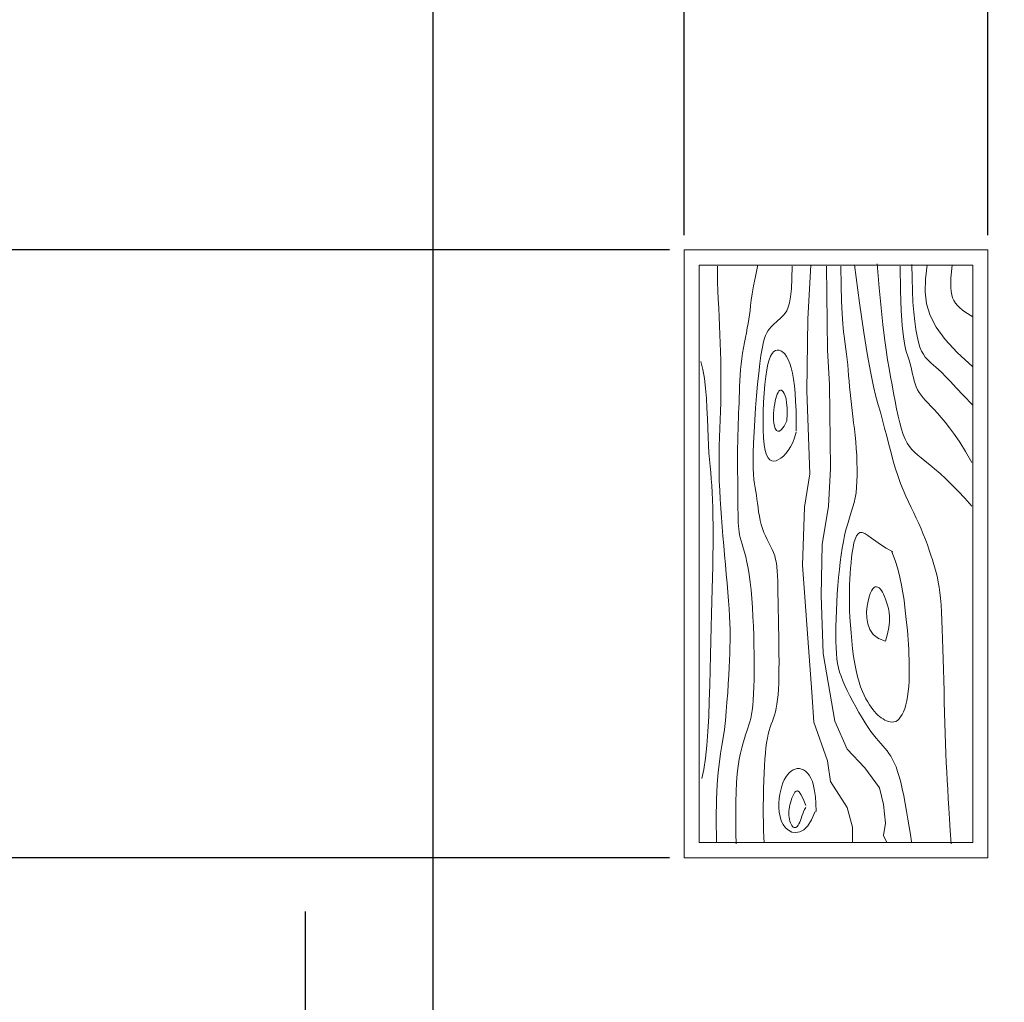
# Model space of a CAD drawing. Units: inches. Extents: x 2923 to 3500, y 1684 to 2381.
# Tile 5 of 12: x 3176 to 3218, y 1888 to 1930. Entities that reach past the tile are written whole.
import ezdxf

# ---------------------------------------------------------------- set-up
doc = ezdxf.new("R2010")
doc.units = ezdxf.units.IN
doc.layers.add('A-ANNO-DIMS', color=2, linetype='Continuous', lineweight=18)
doc.layers.add('Furniture', color=7, linetype='Continuous', lineweight=15)
doc.styles.get("Standard").update_dxf_attribs({"font": 'txt', "height": 5})
doc.dimstyles.new('ISO-25', dxfattribs={"dimtxt": 5, "dimasz": 2.5, "dimexe": 1.25, "dimexo": 0.625, "dimtad": 1, "dimlunit": 3, "dimtxsty": 'Standard', "dimcen": 2.5, "dimadec": 0, "dimazin": 0, "dimtfac": 1, "dimtmove": 0, "dimatfit": 3, "dimfxl": 1, "dimarcsym": 0})

# ---------------------------------------------------------------- blocks, each defined once
blk = doc.blocks.new('*D30')
at = {"layer": 'A-ANNO-DIMS', "color": 0, "lineweight": -2, "transparency": 16777216}
for p, q in [((3188.23, 1847.406), (3188.23, 1891.632)), ((3179.855, 1847.406), (3189.48, 1847.406)), ((3188.23, 1819.906), (3188.23, 1844.906)), ((3179.855, 1817.406), (3189.48, 1817.406))]:
    blk.add_line(p, q, dxfattribs=at)
at = {"layer": 'A-ANNO-DIMS', "color": 0, "transparency": 16777216}
for points in [[(3187.813, 1844.906), (3188.646, 1844.906), (3188.23, 1847.406)], [(3187.813, 1819.906), (3188.646, 1819.906), (3188.23, 1817.406)]]:
    blk.add_solid(points, dxfattribs=at)
at = {"layer": 'Defpoints', "color": 0, "transparency": 16777216}
for p in [(3179.23, 1847.406), (3188.23, 1847.406), (3179.23, 1817.406)]:
    blk.add_point(p, dxfattribs=at)
at = {"layer": 'A-ANNO-DIMS', "color": 0, "transparency": 16777216, "insert": (3184.629, 1870.769), "char_height": 5, "attachment_point": 5, "rotation": 90}
blk.add_mtext('2\'-6" TYP.', dxfattribs=at)
blk = doc.blocks.new('*D54')
at = {"layer": 'A-ANNO-DIMS', "color": 0, "lineweight": -2, "transparency": 16777216}
for p, q in [((3166.316, 2236.755), (3166.316, 1685.656)), ((3193.644, 2236.755), (3193.644, 1685.656)), ((3168.816, 1686.906), (3191.144, 1686.906)), ((3193.644, 1686.906), (3235.489, 1686.906))]:
    blk.add_line(p, q, dxfattribs=at)
at = {"layer": 'A-ANNO-DIMS', "color": 0, "transparency": 16777216}
for points in [[(3168.816, 1687.323), (3168.816, 1686.49), (3166.316, 1686.906)], [(3191.144, 1687.323), (3191.144, 1686.49), (3193.644, 1686.906)]]:
    blk.add_solid(points, dxfattribs=at)
at = {"layer": 'Defpoints', "color": 0, "transparency": 16777216}
for p in [(3166.316, 2237.38), (3193.644, 2237.38), (3193.644, 1686.906)]:
    blk.add_point(p, dxfattribs=at)
at = {"layer": 'A-ANNO-DIMS', "color": 0, "transparency": 16777216, "insert": (3215.817, 1691.341), "char_height": 5, "attachment_point": 5}
blk.add_mtext('2\'-3 1/2"', dxfattribs=at)
blk = doc.blocks.new('*D62')
at = {"layer": 'A-ANNO-DIMS', "color": 0, "lineweight": -2, "transparency": 16777216}
for p, q in [((3204.334, 1920.391), (3204.334, 2370.156)), ((3217.261, 1920.391), (3217.261, 2370.156)), ((3206.834, 2368.906), (3214.761, 2368.906)), ((3217.261, 2368.906), (3238.868, 2368.906))]:
    blk.add_line(p, q, dxfattribs=at)
at = {"layer": 'A-ANNO-DIMS', "color": 0, "transparency": 16777216}
for points in [[(3206.834, 2369.323), (3206.834, 2368.49), (3204.334, 2368.906)], [(3214.761, 2369.323), (3214.761, 2368.49), (3217.261, 2368.906)]]:
    blk.add_solid(points, dxfattribs=at)
at = {"layer": 'Defpoints', "color": 0, "transparency": 16777216}
for p in [(3217.261, 2368.906), (3204.334, 1919.766), (3217.261, 1919.766)]:
    blk.add_point(p, dxfattribs=at)
at = {"layer": 'A-ANNO-DIMS', "color": 0, "transparency": 16777216, "insert": (3229.315, 2372.507), "char_height": 5, "attachment_point": 5}
blk.add_mtext('1\'-1"', dxfattribs=at)
blk = doc.blocks.new('*D63')
at = {"layer": 'A-ANNO-DIMS', "color": 0, "lineweight": -2, "transparency": 16777216}
for p, q in [((3203.709, 1919.766), (2933.48, 1919.766)), ((2934.73, 1896.412), (2934.73, 1917.266)), ((3203.709, 1893.912), (2933.48, 1893.912))]:
    blk.add_line(p, q, dxfattribs=at)
at = {"layer": 'A-ANNO-DIMS', "color": 0, "transparency": 16777216}
for points in [[(2934.313, 1917.266), (2935.146, 1917.266), (2934.73, 1919.766)], [(2934.313, 1896.412), (2935.146, 1896.412), (2934.73, 1893.912)]]:
    blk.add_solid(points, dxfattribs=at)
at = {"layer": 'Defpoints', "color": 0, "transparency": 16777216}
for p in [(2934.73, 1919.766), (3204.334, 1919.766), (3204.334, 1893.912)]:
    blk.add_point(p, dxfattribs=at)
at = {"layer": 'A-ANNO-DIMS', "color": 0, "transparency": 16777216, "insert": (2931.129, 1906.839), "char_height": 5, "attachment_point": 5, "rotation": 90}
blk.add_mtext('2\'-2"', dxfattribs=at)
blk = doc.blocks.new('*D65')
at = {"layer": 'A-ANNO-DIMS', "color": 0, "lineweight": -2, "transparency": 16777216}
for p, q in [((2934.73, 1882.852), (2934.73, 1905.411)), ((3193.074, 1882.852), (2933.48, 1882.852)), ((2934.73, 1868.288), (2934.73, 1880.352)), ((3193.074, 1865.788), (2933.48, 1865.788))]:
    blk.add_line(p, q, dxfattribs=at)
at = {"layer": 'A-ANNO-DIMS', "color": 0, "transparency": 16777216}
for points in [[(2934.313, 1880.352), (2935.146, 1880.352), (2934.73, 1882.852)], [(2934.313, 1868.288), (2935.146, 1868.288), (2934.73, 1865.788)]]:
    blk.add_solid(points, dxfattribs=at)
at = {"layer": 'Defpoints', "color": 0, "transparency": 16777216}
for p in [(2934.73, 1882.852), (3193.699, 1882.852), (3193.699, 1865.788)]:
    blk.add_point(p, dxfattribs=at)
at = {"layer": 'A-ANNO-DIMS', "color": 0, "transparency": 16777216, "insert": (2931.129, 1895.382), "char_height": 5, "attachment_point": 5, "rotation": 90}
blk.add_mtext('1\'-5"', dxfattribs=at)

msp = doc.modelspace()

# ---------------------------------------------------------------- linework, layer by layer
at = {"layer": 'Furniture'}
for p, q in [((3204.334, 1893.912), (3204.334, 1919.766)), ((3204.334, 1919.766), (3217.261, 1919.766)), ((3217.261, 1919.766), (3217.261, 1893.912)), ((3204.981, 1894.558), (3204.981, 1919.119)), ((3204.981, 1919.119), (3216.615, 1919.119)), ((3205.753, 1919.085), (3205.756, 1918.746)), ((3207.476, 1919.129), (3207.374, 1918.644)), ((3208.934, 1919.085), (3208.926, 1918.547)), ((3209.73, 1919.129), (3209.597, 1916.83)), ((3210.393, 1919.085), (3210.437, 1915.504)), ((3211.011, 1919.085), (3211.017, 1918.258)), ((3211.586, 1919.129), (3211.801, 1917.524)), ((3212.558, 1919.173), (3212.639, 1918.155)), ((3213.53, 1919.085), (3213.541, 1918.029)), ((3214.031, 1919.144), (3214.036, 1918.562)), ((3214.679, 1919.129), (3214.605, 1918.531)), ((3215.739, 1919.129), (3215.71, 1918.835)), ((3216.615, 1919.119), (3216.615, 1894.558)), ((3205.756, 1918.746), (3205.764, 1918.396)), ((3207.374, 1918.644), (3207.296, 1918.241)), ((3208.926, 1918.547), (3208.904, 1918.116)), ((3214.036, 1918.562), (3214.05, 1918.03)), ((3214.605, 1918.531), (3214.591, 1917.986)), ((3215.691, 1918.58), (3215.681, 1918.359)), ((3215.71, 1918.835), (3215.691, 1918.58)), ((3205.764, 1918.396), (3205.776, 1918.035)), ((3207.296, 1918.241), (3207.238, 1917.908)), ((3208.904, 1918.116), (3208.868, 1917.779)), ((3211.017, 1918.258), (3211.033, 1917.587)), ((3212.639, 1918.155), (3212.716, 1917.305)), ((3215.681, 1918.359), (3215.683, 1918.169)), ((3215.683, 1918.169), (3215.696, 1918.004)), ((3205.776, 1918.035), (3205.791, 1917.668)), ((3205.791, 1917.668), (3205.808, 1917.295)), ((3207.196, 1917.631), (3207.165, 1917.398)), ((3207.238, 1917.908), (3207.196, 1917.631)), ((3208.868, 1917.779), (3208.821, 1917.521)), ((3213.541, 1918.029), (3213.57, 1917.194)), ((3214.05, 1918.03), (3214.074, 1917.548)), ((3214.591, 1917.986), (3214.653, 1917.475)), ((3215.696, 1918.004), (3215.722, 1917.859)), ((3215.722, 1917.859), (3215.762, 1917.731)), ((3215.762, 1917.731), (3215.817, 1917.615)), ((3205.808, 1917.295), (3205.826, 1916.92)), ((3207.165, 1917.398), (3207.141, 1917.196)), ((3208.765, 1917.328), (3208.701, 1917.184)), ((3208.821, 1917.521), (3208.765, 1917.328)), ((3211.033, 1917.587), (3211.057, 1917.049)), ((3211.801, 1917.524), (3211.985, 1916.255)), ((3212.716, 1917.305), (3212.79, 1916.598)), ((3214.074, 1917.548), (3214.107, 1917.115)), ((3214.653, 1917.475), (3214.806, 1916.979)), ((3215.817, 1917.615), (3215.886, 1917.506)), ((3215.886, 1917.506), (3215.969, 1917.405)), ((3215.969, 1917.405), (3216.063, 1917.31)), ((3216.063, 1917.31), (3216.166, 1917.221)), ((3216.166, 1917.221), (3216.276, 1917.138)), ((3205.826, 1916.92), (3205.843, 1916.544)), ((3207.093, 1916.83), (3207.062, 1916.644)), ((3207.118, 1917.01), (3207.093, 1916.83)), ((3207.141, 1917.196), (3207.118, 1917.01)), ((3208.407, 1916.837), (3208.33, 1916.767)), ((3208.483, 1916.91), (3208.407, 1916.837)), ((3208.559, 1916.989), (3208.483, 1916.91)), ((3208.632, 1917.076), (3208.559, 1916.989)), ((3208.701, 1917.184), (3208.632, 1917.076)), ((3209.597, 1916.83), (3209.553, 1913.78)), ((3211.057, 1917.049), (3211.088, 1916.62)), ((3213.57, 1917.194), (3213.614, 1916.55)), ((3214.107, 1917.115), (3214.147, 1916.729)), ((3214.806, 1916.979), (3215.064, 1916.482)), ((3216.276, 1917.138), (3216.39, 1917.06)), ((3216.39, 1917.06), (3216.506, 1916.987)), ((3216.506, 1916.987), (3216.623, 1916.919)), ((3205.843, 1916.544), (3205.86, 1916.171)), ((3207.026, 1916.449), (3206.987, 1916.248)), ((3207.062, 1916.644), (3207.026, 1916.449)), ((3207.97, 1916.417), (3207.908, 1916.336)), ((3208.035, 1916.492), (3207.97, 1916.417)), ((3208.105, 1916.563), (3208.035, 1916.492)), ((3208.178, 1916.632), (3208.105, 1916.563)), ((3208.253, 1916.699), (3208.178, 1916.632)), ((3208.33, 1916.767), (3208.253, 1916.699)), ((3211.088, 1916.62), (3211.122, 1916.279)), ((3212.79, 1916.598), (3212.861, 1916.012)), ((3213.614, 1916.55), (3213.668, 1916.065)), ((3214.147, 1916.729), (3214.194, 1916.39)), ((3214.194, 1916.39), (3214.247, 1916.096)), ((3215.064, 1916.482), (3215.443, 1915.965)), ((3205.86, 1916.171), (3205.874, 1915.801)), ((3206.945, 1916.04), (3206.903, 1915.825)), ((3206.987, 1916.248), (3206.945, 1916.04)), ((3207.747, 1915.978), (3207.698, 1915.794)), ((3207.798, 1916.124), (3207.747, 1915.978)), ((3207.851, 1916.241), (3207.798, 1916.124)), ((3207.908, 1916.336), (3207.851, 1916.241)), ((3211.122, 1916.279), (3211.157, 1916.001)), ((3211.157, 1916.001), (3211.192, 1915.765)), ((3211.985, 1916.255), (3212.143, 1915.272)), ((3212.861, 1916.012), (3212.929, 1915.52)), ((3213.668, 1916.065), (3213.729, 1915.707)), ((3214.247, 1916.096), (3214.307, 1915.846)), ((3215.443, 1915.965), (3215.958, 1915.409)), ((3205.874, 1915.801), (3205.885, 1915.435)), ((3206.862, 1915.605), (3206.824, 1915.38)), ((3206.903, 1915.825), (3206.862, 1915.605)), ((3207.651, 1915.565), (3207.604, 1915.281)), ((3207.698, 1915.794), (3207.651, 1915.565)), ((3211.192, 1915.765), (3211.225, 1915.548)), ((3211.225, 1915.548), (3211.253, 1915.33)), ((3213.729, 1915.707), (3213.792, 1915.445)), ((3214.307, 1915.846), (3214.371, 1915.639)), ((3214.371, 1915.639), (3214.441, 1915.469)), ((3205.885, 1915.435), (3205.894, 1915.072)), ((3206.791, 1915.15), (3206.764, 1914.916)), ((3206.824, 1915.38), (3206.791, 1915.15)), ((3207.604, 1915.281), (3207.557, 1914.936)), ((3208.018, 1915.249), (3207.958, 1915.097)), ((3208.083, 1915.362), (3208.018, 1915.249)), ((3208.152, 1915.442), (3208.083, 1915.362)), ((3208.225, 1915.49), (3208.152, 1915.442)), ((3208.301, 1915.511), (3208.225, 1915.49)), ((3208.379, 1915.507), (3208.301, 1915.511)), ((3208.459, 1915.479), (3208.379, 1915.507)), ((3208.539, 1915.424), (3208.459, 1915.479)), ((3208.618, 1915.344), (3208.539, 1915.424)), ((3208.694, 1915.237), (3208.618, 1915.344)), ((3208.766, 1915.102), (3208.694, 1915.237)), ((3210.437, 1915.504), (3210.525, 1914.045)), ((3211.253, 1915.33), (3211.277, 1915.109)), ((3212.143, 1915.272), (3212.278, 1914.524)), ((3212.929, 1915.52), (3212.996, 1915.1)), ((3213.792, 1915.445), (3213.854, 1915.248)), ((3213.854, 1915.248), (3213.909, 1915.084)), ((3214.441, 1915.469), (3214.516, 1915.329)), ((3214.516, 1915.329), (3214.594, 1915.213)), ((3214.594, 1915.213), (3214.678, 1915.116)), ((3214.678, 1915.116), (3214.765, 1915.03)), ((3215.958, 1915.409), (3216.623, 1914.796)), ((3205.046, 1915.017), (3205.133, 1914.678)), ((3205.894, 1915.072), (3205.9, 1914.711)), ((3205.9, 1914.711), (3205.903, 1914.351)), ((3206.764, 1914.916), (3206.742, 1914.679)), ((3207.557, 1914.936), (3207.51, 1914.526)), ((3207.902, 1914.905), (3207.852, 1914.668)), ((3207.958, 1915.097), (3207.902, 1914.905)), ((3208.833, 1914.94), (3208.766, 1915.102)), ((3208.894, 1914.749), (3208.833, 1914.94)), ((3208.946, 1914.528), (3208.894, 1914.749)), ((3211.277, 1915.109), (3211.299, 1914.883)), ((3211.299, 1914.883), (3211.319, 1914.654)), ((3212.996, 1915.1), (3213.061, 1914.725)), ((3213.061, 1914.725), (3213.125, 1914.373)), ((3213.909, 1915.084), (3213.956, 1914.927)), ((3213.956, 1914.927), (3213.995, 1914.774)), ((3213.995, 1914.774), (3214.029, 1914.623)), ((3214.765, 1915.03), (3214.856, 1914.951)), ((3214.856, 1914.951), (3214.951, 1914.87)), ((3214.951, 1914.87), (3215.051, 1914.782)), ((3215.051, 1914.782), (3215.163, 1914.678)), ((3205.133, 1914.678), (3205.2, 1914.299)), ((3205.2, 1914.299), (3205.249, 1913.89)), ((3205.903, 1914.351), (3205.903, 1913.992)), ((3206.724, 1914.441), (3206.71, 1914.202)), ((3206.742, 1914.679), (3206.724, 1914.441)), ((3207.51, 1914.526), (3207.464, 1914.063)), ((3207.808, 1914.384), (3207.769, 1914.051)), ((3207.852, 1914.668), (3207.808, 1914.384)), ((3208.991, 1914.276), (3208.946, 1914.528)), ((3209.029, 1913.993), (3208.991, 1914.276)), ((3211.319, 1914.654), (3211.338, 1914.42)), ((3211.338, 1914.42), (3211.357, 1914.183)), ((3212.278, 1914.524), (3212.396, 1913.96)), ((3213.125, 1914.373), (3213.188, 1914.023)), ((3214.029, 1914.623), (3214.061, 1914.477)), ((3214.061, 1914.477), (3214.092, 1914.335)), ((3214.092, 1914.335), (3214.127, 1914.198)), ((3215.163, 1914.678), (3215.297, 1914.548)), ((3215.297, 1914.548), (3215.462, 1914.382)), ((3215.462, 1914.382), (3215.666, 1914.171)), ((3205.249, 1913.89), (3205.283, 1913.464)), ((3205.903, 1913.992), (3205.899, 1913.632)), ((3206.699, 1913.965), (3206.69, 1913.73)), ((3206.71, 1914.202), (3206.699, 1913.965)), ((3207.464, 1914.063), (3207.419, 1913.564)), ((3207.769, 1914.051), (3207.738, 1913.681)), ((3209.059, 1913.677), (3209.029, 1913.993)), ((3210.525, 1914.045), (3210.569, 1910.464)), ((3211.357, 1914.183), (3211.378, 1913.943)), ((3211.378, 1913.943), (3211.401, 1913.699)), ((3212.396, 1913.96), (3212.501, 1913.529)), ((3213.188, 1914.023), (3213.251, 1913.675)), ((3214.127, 1914.198), (3214.167, 1914.067)), ((3214.167, 1914.067), (3214.215, 1913.942)), ((3214.215, 1913.942), (3214.272, 1913.823)), ((3215.666, 1914.171), (3215.919, 1913.906)), ((3215.919, 1913.906), (3216.23, 1913.578)), ((3205.283, 1913.464), (3205.308, 1913.031)), ((3205.899, 1913.632), (3205.893, 1913.271)), ((3206.681, 1913.498), (3206.673, 1913.271)), ((3206.69, 1913.73), (3206.681, 1913.498)), ((3207.419, 1913.564), (3207.379, 1913.046)), ((3207.738, 1913.681), (3207.715, 1913.289)), ((3208.242, 1913.455), (3208.215, 1913.344)), ((3208.27, 1913.553), (3208.242, 1913.455)), ((3208.3, 1913.637), (3208.27, 1913.553)), ((3208.332, 1913.704), (3208.3, 1913.637)), ((3208.364, 1913.756), (3208.332, 1913.704)), ((3208.399, 1913.79), (3208.364, 1913.756)), ((3208.436, 1913.806), (3208.399, 1913.79)), ((3208.474, 1913.803), (3208.436, 1913.806)), ((3208.515, 1913.78), (3208.474, 1913.803)), ((3208.557, 1913.735), (3208.515, 1913.78)), ((3208.598, 1913.666), (3208.557, 1913.735)), ((3208.638, 1913.568), (3208.598, 1913.666)), ((3208.672, 1913.437), (3208.638, 1913.568)), ((3208.699, 1913.268), (3208.672, 1913.437)), ((3209.082, 1913.326), (3209.059, 1913.677)), ((3209.553, 1913.78), (3209.686, 1910.243)), ((3211.401, 1913.699), (3211.428, 1913.451)), ((3211.428, 1913.451), (3211.457, 1913.199)), ((3212.501, 1913.529), (3212.596, 1913.18)), ((3213.251, 1913.675), (3213.315, 1913.335)), ((3214.272, 1913.823), (3214.34, 1913.709)), ((3214.34, 1913.709), (3214.419, 1913.597)), ((3214.419, 1913.597), (3214.508, 1913.484)), ((3214.508, 1913.484), (3214.608, 1913.368)), ((3216.23, 1913.578), (3216.608, 1913.175)), ((3205.308, 1913.031), (3205.325, 1912.604)), ((3205.893, 1913.271), (3205.883, 1912.908)), ((3206.665, 1913.05), (3206.656, 1912.831)), ((3206.673, 1913.271), (3206.665, 1913.05)), ((3207.379, 1913.046), (3207.343, 1912.528)), ((3207.715, 1913.289), (3207.701, 1912.887)), ((3208.17, 1913.09), (3208.154, 1912.953)), ((3208.191, 1913.221), (3208.17, 1913.09)), ((3208.215, 1913.344), (3208.191, 1913.221)), ((3208.716, 1913.058), (3208.699, 1913.268)), ((3208.722, 1912.803), (3208.716, 1913.058)), ((3209.098, 1912.94), (3209.082, 1913.326)), ((3211.457, 1913.199), (3211.488, 1912.944)), ((3212.596, 1913.18), (3212.687, 1912.862)), ((3213.315, 1913.335), (3213.38, 1913.007)), ((3214.608, 1913.368), (3214.719, 1913.246)), ((3214.719, 1913.246), (3214.841, 1913.117)), ((3214.841, 1913.117), (3214.973, 1912.976)), ((3205.325, 1912.604), (3205.34, 1912.192)), ((3205.883, 1912.908), (3205.871, 1912.543)), ((3206.647, 1912.609), (3206.638, 1912.382)), ((3206.656, 1912.831), (3206.647, 1912.609)), ((3207.701, 1912.887), (3207.696, 1912.491)), ((3208.144, 1912.813), (3208.14, 1912.673)), ((3208.14, 1912.673), (3208.144, 1912.535)), ((3208.154, 1912.953), (3208.144, 1912.813)), ((3208.713, 1912.498), (3208.722, 1912.803)), ((3209.108, 1912.517), (3209.098, 1912.94)), ((3211.488, 1912.944), (3211.519, 1912.685)), ((3211.519, 1912.685), (3211.551, 1912.42)), ((3212.687, 1912.862), (3212.776, 1912.534)), ((3213.38, 1913.007), (3213.446, 1912.697)), ((3213.446, 1912.697), (3213.515, 1912.408)), ((3214.973, 1912.976), (3215.117, 1912.822)), ((3215.117, 1912.822), (3215.274, 1912.647)), ((3215.274, 1912.647), (3215.445, 1912.444)), ((3205.34, 1912.192), (3205.355, 1911.809)), ((3205.871, 1912.543), (3205.858, 1912.176)), ((3206.638, 1912.382), (3206.631, 1912.145)), ((3207.343, 1912.528), (3207.313, 1912.025)), ((3207.696, 1912.491), (3207.702, 1912.114)), ((3208.144, 1912.535), (3208.157, 1912.402)), ((3208.157, 1912.402), (3208.18, 1912.277)), ((3208.18, 1912.277), (3208.215, 1912.171)), ((3208.484, 1912.135), (3208.59, 1912.276)), ((3208.59, 1912.276), (3208.713, 1912.498)), ((3209.111, 1912.055), (3209.108, 1912.517)), ((3211.551, 1912.42), (3211.582, 1912.152)), ((3212.776, 1912.534), (3212.866, 1912.192)), ((3212.866, 1912.192), (3212.957, 1911.84)), ((3213.515, 1912.408), (3213.587, 1912.146)), ((3215.445, 1912.444), (3215.632, 1912.204)), ((3215.632, 1912.204), (3215.838, 1911.92)), ((3205.355, 1911.809), (3205.374, 1911.461)), ((3205.846, 1911.807), (3205.835, 1911.435)), ((3205.858, 1912.176), (3205.846, 1911.807)), ((3206.624, 1911.894), (3206.618, 1911.625)), ((3206.631, 1912.145), (3206.624, 1911.894)), ((3207.313, 1912.025), (3207.291, 1911.555)), ((3207.702, 1912.114), (3207.719, 1911.77)), ((3207.719, 1911.77), (3207.749, 1911.473)), ((3208.215, 1912.171), (3208.261, 1912.093)), ((3208.261, 1912.093), (3208.321, 1912.055)), ((3208.321, 1912.055), (3208.395, 1912.065)), ((3208.395, 1912.065), (3208.484, 1912.135)), ((3208.956, 1911.57), (3209.039, 1911.777)), ((3209.039, 1911.777), (3209.111, 1912.011)), ((3211.582, 1912.152), (3211.611, 1911.878)), ((3211.611, 1911.878), (3211.637, 1911.599)), ((3212.957, 1911.84), (3213.049, 1911.485)), ((3213.587, 1912.146), (3213.662, 1911.915)), ((3213.662, 1911.915), (3213.742, 1911.72)), ((3215.838, 1911.92), (3216.063, 1911.585)), ((3205.374, 1911.461), (3205.395, 1911.144)), ((3205.835, 1911.435), (3205.828, 1911.062)), ((3206.618, 1911.625), (3206.614, 1911.333)), ((3207.291, 1911.555), (3207.277, 1911.134)), ((3207.749, 1911.473), (3207.791, 1911.235)), ((3208.768, 1911.236), (3208.865, 1911.39)), ((3208.865, 1911.39), (3208.956, 1911.57)), ((3211.637, 1911.599), (3211.66, 1911.315)), ((3213.049, 1911.485), (3213.143, 1911.131)), ((3213.742, 1911.72), (3213.828, 1911.554)), ((3213.828, 1911.554), (3213.923, 1911.41)), ((3213.923, 1911.41), (3214.028, 1911.282)), ((3216.063, 1911.585), (3216.309, 1911.19)), ((3205.395, 1911.144), (3205.419, 1910.85)), ((3205.828, 1911.062), (3205.824, 1910.687)), ((3206.614, 1911.333), (3206.613, 1911.018)), ((3206.613, 1911.018), (3206.613, 1910.684)), ((3207.277, 1911.134), (3207.274, 1910.777)), ((3207.791, 1911.235), (3207.845, 1911.053)), ((3207.845, 1911.053), (3207.91, 1910.922)), ((3207.91, 1910.922), (3207.984, 1910.837)), ((3208.456, 1910.912), (3208.561, 1910.998)), ((3208.561, 1910.998), (3208.666, 1911.105)), ((3208.666, 1911.105), (3208.768, 1911.236)), ((3211.66, 1911.315), (3211.679, 1911.028)), ((3211.679, 1911.028), (3211.692, 1910.743)), ((3213.143, 1911.131), (3213.239, 1910.784)), ((3214.028, 1911.282), (3214.146, 1911.163)), ((3214.146, 1911.163), (3214.279, 1911.045)), ((3214.279, 1911.045), (3214.428, 1910.921)), ((3214.428, 1910.921), (3214.598, 1910.784)), ((3216.309, 1911.19), (3216.579, 1910.729)), ((3205.419, 1910.85), (3205.444, 1910.572)), ((3205.444, 1910.572), (3205.468, 1910.301)), ((3205.824, 1910.687), (3205.826, 1910.309)), ((3206.613, 1910.684), (3206.614, 1910.341)), ((3207.274, 1910.777), (3207.279, 1910.476)), ((3207.984, 1910.837), (3208.067, 1910.792)), ((3208.067, 1910.792), (3208.157, 1910.782)), ((3208.157, 1910.782), (3208.252, 1910.802)), ((3208.252, 1910.802), (3208.353, 1910.847)), ((3208.353, 1910.847), (3208.456, 1910.912)), ((3211.692, 1910.743), (3211.7, 1910.461)), ((3213.239, 1910.784), (3213.338, 1910.45)), ((3214.598, 1910.784), (3214.788, 1910.629)), ((3214.788, 1910.629), (3214.997, 1910.453)), ((3205.468, 1910.301), (3205.492, 1910.03)), ((3205.826, 1910.309), (3205.835, 1909.93)), ((3206.614, 1910.341), (3206.616, 1909.996)), ((3207.279, 1910.476), (3207.292, 1910.224)), ((3207.292, 1910.224), (3207.31, 1910.009)), ((3209.686, 1910.243), (3209.465, 1908.828)), ((3210.569, 1910.464), (3210.481, 1908.872)), ((3211.7, 1910.187), (3211.693, 1909.923)), ((3211.7, 1910.461), (3211.7, 1910.187)), ((3213.338, 1910.45), (3213.441, 1910.132)), ((3213.441, 1910.132), (3213.548, 1909.836)), ((3214.997, 1910.453), (3215.225, 1910.254)), ((3215.225, 1910.254), (3215.469, 1910.031)), ((3205.492, 1910.03), (3205.513, 1909.75)), ((3205.513, 1909.75), (3205.532, 1909.454)), ((3205.835, 1909.93), (3205.85, 1909.548)), ((3206.616, 1909.996), (3206.619, 1909.658)), ((3207.31, 1910.009), (3207.333, 1909.823)), ((3207.333, 1909.823), (3207.358, 1909.655)), ((3211.677, 1909.673), (3211.652, 1909.44)), ((3211.693, 1909.923), (3211.677, 1909.673)), ((3213.548, 1909.836), (3213.658, 1909.56)), ((3215.469, 1910.031), (3215.729, 1909.783)), ((3215.729, 1909.783), (3216.001, 1909.508)), ((3205.532, 1909.454), (3205.546, 1909.136)), ((3205.85, 1909.548), (3205.871, 1909.163)), ((3206.619, 1909.658), (3206.623, 1909.336)), ((3206.623, 1909.336), (3206.626, 1909.037)), ((3207.358, 1909.655), (3207.384, 1909.496)), ((3207.384, 1909.496), (3207.41, 1909.337)), ((3207.41, 1909.337), (3207.434, 1909.169)), ((3211.652, 1909.44), (3211.617, 1909.225)), ((3213.658, 1909.56), (3213.77, 1909.3)), ((3213.77, 1909.3), (3213.882, 1909.054)), ((3216.001, 1909.508), (3216.285, 1909.205)), ((3205.546, 1909.136), (3205.557, 1908.794)), ((3205.871, 1909.163), (3205.896, 1908.776)), ((3206.626, 1909.037), (3206.629, 1908.769)), ((3207.434, 1909.169), (3207.457, 1908.993)), ((3207.457, 1908.993), (3207.482, 1908.812)), ((3209.465, 1908.828), (3209.376, 1906.352)), ((3210.481, 1908.872), (3210.216, 1907.237)), ((3211.522, 1908.835), (3211.466, 1908.65)), ((3211.573, 1909.025), (3211.522, 1908.835)), ((3211.617, 1909.225), (3211.573, 1909.025)), ((3213.882, 1909.054), (3213.995, 1908.817)), ((3216.285, 1909.205), (3216.579, 1908.872)), ((3205.557, 1908.794), (3205.564, 1908.43)), ((3205.564, 1908.43), (3205.568, 1908.044)), ((3205.896, 1908.776), (3205.924, 1908.385)), ((3206.629, 1908.769), (3206.632, 1908.54)), ((3206.632, 1908.54), (3206.635, 1908.344)), ((3207.482, 1908.812), (3207.508, 1908.628)), ((3207.508, 1908.628), (3207.539, 1908.444)), ((3207.539, 1908.444), (3207.575, 1908.262)), ((3211.406, 1908.465), (3211.345, 1908.274)), ((3211.466, 1908.65), (3211.406, 1908.465)), ((3213.995, 1908.817), (3214.105, 1908.587)), ((3214.105, 1908.587), (3214.213, 1908.361)), ((3205.568, 1908.044), (3205.568, 1907.638)), ((3205.924, 1908.385), (3205.956, 1907.991)), ((3205.956, 1907.991), (3205.99, 1907.594)), ((3206.635, 1908.344), (3206.639, 1908.175)), ((3206.639, 1908.175), (3206.647, 1908.029)), ((3206.647, 1908.029), (3206.658, 1907.897)), ((3207.575, 1908.262), (3207.617, 1908.085)), ((3207.617, 1908.085), (3207.668, 1907.914)), ((3211.284, 1908.073), (3211.225, 1907.856)), ((3211.345, 1908.274), (3211.284, 1908.073)), ((3214.213, 1908.361), (3214.318, 1908.136)), ((3214.318, 1908.136), (3214.418, 1907.908)), ((3205.568, 1907.638), (3205.566, 1907.213)), ((3205.99, 1907.594), (3206.025, 1907.192)), ((3206.658, 1907.897), (3206.674, 1907.774)), ((3206.674, 1907.774), (3206.696, 1907.655)), ((3206.696, 1907.655), (3206.725, 1907.531)), ((3207.668, 1907.914), (3207.727, 1907.753)), ((3207.727, 1907.753), (3207.794, 1907.6)), ((3207.794, 1907.6), (3207.865, 1907.453)), ((3211.168, 1907.619), (3211.116, 1907.363)), ((3211.225, 1907.856), (3211.168, 1907.619)), ((3211.611, 1907.467), (3211.669, 1907.601)), ((3211.669, 1907.601), (3211.737, 1907.695)), ((3211.737, 1907.695), (3211.818, 1907.745)), ((3211.818, 1907.745), (3211.912, 1907.745)), ((3211.912, 1907.745), (3212.023, 1907.701)), ((3212.023, 1907.701), (3212.154, 1907.62)), ((3212.154, 1907.62), (3212.308, 1907.51)), ((3214.418, 1907.908), (3214.512, 1907.679)), ((3214.512, 1907.679), (3214.602, 1907.451)), ((3205.566, 1907.213), (3205.561, 1906.769)), ((3206.025, 1907.192), (3206.061, 1906.788)), ((3206.725, 1907.531), (3206.762, 1907.399)), ((3206.762, 1907.399), (3206.805, 1907.254)), ((3206.805, 1907.254), (3206.854, 1907.093)), ((3207.865, 1907.453), (3207.937, 1907.31)), ((3207.937, 1907.31), (3208.009, 1907.17)), ((3208.009, 1907.17), (3208.077, 1907.032)), ((3210.216, 1907.237), (3210.172, 1905.07)), ((3211.116, 1907.363), (3211.067, 1907.089)), ((3211.523, 1907.112), (3211.563, 1907.302)), ((3211.563, 1907.302), (3211.611, 1907.467)), ((3212.308, 1907.51), (3212.488, 1907.378)), ((3212.488, 1907.378), (3212.698, 1907.232)), ((3212.698, 1907.232), (3212.941, 1907.079)), ((3214.602, 1907.451), (3214.686, 1907.226)), ((3214.686, 1907.226), (3214.765, 1907.004)), ((3205.561, 1906.769), (3205.554, 1906.308)), ((3206.061, 1906.788), (3206.097, 1906.383)), ((3206.854, 1907.093), (3206.905, 1906.914)), ((3206.905, 1906.914), (3206.958, 1906.714)), ((3208.077, 1907.032), (3208.138, 1906.892)), ((3208.138, 1906.892), (3208.19, 1906.75)), ((3208.19, 1906.75), (3208.232, 1906.604)), ((3211.021, 1906.798), (3210.98, 1906.492)), ((3211.067, 1907.089), (3211.021, 1906.798)), ((3211.462, 1906.682), (3211.49, 1906.903)), ((3211.49, 1906.903), (3211.523, 1907.112)), ((3212.941, 1907.079), (3213.22, 1906.927)), ((3213.176, 1906.927), (3213.312, 1906.564)), ((3214.765, 1907.004), (3214.838, 1906.789)), ((3214.838, 1906.789), (3214.905, 1906.581)), ((3206.097, 1906.383), (3206.133, 1905.982)), ((3206.958, 1906.714), (3207.011, 1906.489)), ((3207.011, 1906.489), (3207.061, 1906.237)), ((3208.232, 1906.604), (3208.263, 1906.449)), ((3208.263, 1906.449), (3208.286, 1906.283)), ((3209.376, 1906.352), (3209.597, 1903.258)), ((3210.98, 1906.492), (3210.942, 1906.173)), ((3211.418, 1906.229), (3211.438, 1906.456)), ((3211.438, 1906.456), (3211.462, 1906.682)), ((3213.312, 1906.564), (3213.425, 1906.205)), ((3214.905, 1906.581), (3214.966, 1906.382)), ((3214.966, 1906.382), (3215.021, 1906.193)), ((3205.554, 1906.308), (3205.545, 1905.83)), ((3206.133, 1905.982), (3206.166, 1905.59)), ((3207.061, 1906.237), (3207.108, 1905.955)), ((3207.108, 1905.955), (3207.149, 1905.64)), ((3208.286, 1906.283), (3208.302, 1906.101)), ((3208.302, 1906.101), (3208.313, 1905.899)), ((3208.313, 1905.899), (3208.32, 1905.674)), ((3210.942, 1906.173), (3210.908, 1905.841)), ((3211.386, 1905.77), (3211.4, 1906.001)), ((3211.4, 1906.001), (3211.418, 1906.229)), ((3213.425, 1906.205), (3213.516, 1905.854)), ((3215.021, 1906.193), (3215.07, 1906.009)), ((3215.07, 1906.009), (3215.114, 1905.824)), ((3205.545, 1905.83), (3205.534, 1905.334)), ((3206.166, 1905.59), (3206.197, 1905.21)), ((3207.149, 1905.64), (3207.186, 1905.298)), ((3208.32, 1905.674), (3208.325, 1905.421)), ((3210.879, 1905.498), (3210.853, 1905.146)), ((3210.908, 1905.841), (3210.879, 1905.498)), ((3211.37, 1905.282), (3211.376, 1905.531)), ((3211.376, 1905.531), (3211.386, 1905.77)), ((3213.516, 1905.854), (3213.589, 1905.513)), ((3213.589, 1905.513), (3213.647, 1905.184)), ((3215.114, 1905.824), (3215.153, 1905.632)), ((3215.153, 1905.632), (3215.187, 1905.427)), ((3205.534, 1905.334), (3205.521, 1904.818)), ((3206.197, 1905.21), (3206.225, 1904.846)), ((3207.186, 1905.298), (3207.217, 1904.934)), ((3208.325, 1905.421), (3208.33, 1905.137)), ((3208.33, 1905.137), (3208.337, 1904.819)), ((3210.172, 1905.07), (3210.26, 1902.595)), ((3210.853, 1905.146), (3210.832, 1904.789)), ((3211.368, 1905.021), (3211.37, 1905.282)), ((3212.257, 1905.157), (3212.209, 1905.012)), ((3212.309, 1905.269), (3212.257, 1905.157)), ((3212.362, 1905.35), (3212.309, 1905.269)), ((3212.417, 1905.403), (3212.362, 1905.35)), ((3212.472, 1905.431), (3212.417, 1905.403)), ((3212.526, 1905.437), (3212.472, 1905.431)), ((3212.58, 1905.424), (3212.526, 1905.437)), ((3212.631, 1905.394), (3212.58, 1905.424)), ((3212.681, 1905.348), (3212.631, 1905.394)), ((3212.729, 1905.287), (3212.681, 1905.348)), ((3212.775, 1905.212), (3212.729, 1905.287)), ((3212.821, 1905.124), (3212.775, 1905.212)), ((3212.865, 1905.024), (3212.821, 1905.124)), ((3213.647, 1905.184), (3213.694, 1904.871)), ((3215.187, 1905.427), (3215.218, 1905.203)), ((3215.218, 1905.203), (3215.244, 1904.953)), ((3205.521, 1904.818), (3205.507, 1904.282)), ((3206.225, 1904.846), (3206.249, 1904.504)), ((3207.217, 1904.934), (3207.243, 1904.553)), ((3208.337, 1904.819), (3208.344, 1904.474)), ((3210.832, 1904.789), (3210.815, 1904.433)), ((3211.371, 1904.745), (3211.368, 1905.021)), ((3211.379, 1904.451), (3211.371, 1904.745)), ((3212.164, 1904.831), (3212.125, 1904.613)), ((3212.209, 1905.012), (3212.164, 1904.831)), ((3212.909, 1904.912), (3212.865, 1905.024)), ((3212.952, 1904.79), (3212.909, 1904.912)), ((3212.994, 1904.658), (3212.952, 1904.79)), ((3213.031, 1904.511), (3212.994, 1904.658)), ((3213.694, 1904.871), (3213.731, 1904.575)), ((3215.244, 1904.953), (3215.268, 1904.672)), ((3215.268, 1904.672), (3215.289, 1904.356)), ((3205.507, 1904.282), (3205.492, 1903.724)), ((3206.249, 1904.504), (3206.268, 1904.186)), ((3207.243, 1904.553), (3207.265, 1904.159)), ((3208.344, 1904.474), (3208.351, 1904.109)), ((3210.815, 1904.433), (3210.803, 1904.083)), ((3211.393, 1904.138), (3211.379, 1904.451)), ((3212.125, 1904.613), (3212.102, 1904.37)), ((3212.102, 1904.37), (3212.105, 1904.115)), ((3213.059, 1904.348), (3213.031, 1904.511)), ((3213.074, 1904.162), (3213.059, 1904.348)), ((3213.731, 1904.575), (3213.762, 1904.3)), ((3213.762, 1904.3), (3213.789, 1904.047)), ((3215.289, 1904.356), (3215.307, 1904.007)), ((3206.268, 1904.186), (3206.282, 1903.895)), ((3206.282, 1903.895), (3206.291, 1903.626)), ((3207.265, 1904.159), (3207.283, 1903.76)), ((3208.351, 1904.109), (3208.358, 1903.731)), ((3210.803, 1904.083), (3210.796, 1903.744)), ((3211.413, 1903.81), (3211.393, 1904.138)), ((3211.438, 1903.474), (3211.413, 1903.81)), ((3212.105, 1904.115), (3212.147, 1903.861)), ((3212.147, 1903.861), (3212.237, 1903.621)), ((3213.045, 1903.711), (3213.071, 1903.951)), ((3213.071, 1903.951), (3213.074, 1904.162)), ((3213.789, 1904.047), (3213.814, 1903.813)), ((3213.814, 1903.813), (3213.835, 1903.594)), ((3215.307, 1904.007), (3215.323, 1903.629)), ((3205.492, 1903.724), (3205.476, 1903.143)), ((3206.291, 1903.626), (3206.295, 1903.369)), ((3207.283, 1903.76), (3207.297, 1903.359)), ((3208.358, 1903.731), (3208.365, 1903.349)), ((3210.796, 1903.744), (3210.794, 1903.421)), ((3210.794, 1903.421), (3210.797, 1903.12)), ((3211.469, 1903.135), (3211.438, 1903.474)), ((3212.237, 1903.621), (3212.387, 1903.41)), ((3212.387, 1903.41), (3212.608, 1903.24)), ((3212.911, 1903.125), (3212.994, 1903.437)), ((3212.994, 1903.437), (3213.045, 1903.711)), ((3213.835, 1903.594), (3213.854, 1903.384)), ((3213.854, 1903.384), (3213.871, 1903.181)), ((3215.323, 1903.629), (3215.338, 1903.226)), ((3205.476, 1903.143), (3205.46, 1902.537)), ((3206.294, 1903.119), (3206.289, 1902.865)), ((3206.295, 1903.369), (3206.294, 1903.119)), ((3207.297, 1903.359), (3207.307, 1902.963)), ((3207.307, 1902.963), (3207.313, 1902.576)), ((3208.365, 1903.349), (3208.37, 1902.969)), ((3208.37, 1902.969), (3208.373, 1902.6)), ((3209.597, 1903.258), (3209.774, 1900.959)), ((3210.797, 1903.12), (3210.805, 1902.845)), ((3211.505, 1902.8), (3211.469, 1903.135)), ((3212.608, 1903.24), (3212.911, 1903.125)), ((3213.871, 1903.181), (3213.885, 1902.98)), ((3213.885, 1902.98), (3213.896, 1902.776)), ((3215.338, 1903.226), (3215.351, 1902.804)), ((3206.281, 1902.602), (3206.269, 1902.32)), ((3206.289, 1902.865), (3206.281, 1902.602)), ((3207.313, 1902.576), (3207.316, 1902.202)), ((3208.373, 1902.6), (3208.375, 1902.248)), ((3210.26, 1902.595), (3210.746, 1899.721)), ((3210.805, 1902.845), (3210.819, 1902.6)), ((3210.819, 1902.6), (3210.84, 1902.381)), ((3211.548, 1902.475), (3211.505, 1902.8)), ((3213.896, 1902.776), (3213.905, 1902.565)), ((3213.905, 1902.565), (3213.913, 1902.345)), ((3215.351, 1902.804), (3215.363, 1902.366)), ((3205.46, 1902.537), (3205.444, 1901.906)), ((3206.269, 1902.32), (3206.254, 1902.012)), ((3207.316, 1902.202), (3207.316, 1901.843)), ((3208.375, 1902.248), (3208.373, 1901.921)), ((3210.84, 1902.381), (3210.868, 1902.181)), ((3210.868, 1902.181), (3210.906, 1901.993)), ((3211.597, 1902.167), (3211.548, 1902.475)), ((3211.652, 1901.88), (3211.597, 1902.167)), ((3213.913, 1902.345), (3213.917, 1902.116)), ((3215.363, 1902.366), (3215.375, 1901.916)), ((3205.444, 1901.906), (3205.427, 1901.25)), ((3206.254, 1902.012), (3206.236, 1901.674)), ((3207.316, 1901.843), (3207.311, 1901.502)), ((3208.373, 1901.921), (3208.369, 1901.618)), ((3210.906, 1901.993), (3210.954, 1901.812)), ((3210.954, 1901.812), (3211.014, 1901.632)), ((3211.713, 1901.62), (3211.652, 1901.88)), ((3213.918, 1901.884), (3213.915, 1901.651)), ((3213.917, 1902.116), (3213.918, 1901.884)), ((3215.375, 1901.916), (3215.386, 1901.46)), ((3206.214, 1901.309), (3206.19, 1900.926)), ((3206.236, 1901.674), (3206.214, 1901.309)), ((3207.311, 1901.502), (3207.303, 1901.183)), ((3208.361, 1901.34), (3208.349, 1901.084)), ((3208.369, 1901.618), (3208.361, 1901.34)), ((3211.014, 1901.632), (3211.087, 1901.445)), ((3211.087, 1901.445), (3211.173, 1901.246)), ((3211.779, 1901.387), (3211.713, 1901.62)), ((3211.849, 1901.177), (3211.779, 1901.387)), ((3213.907, 1901.419), (3213.893, 1901.194)), ((3213.915, 1901.651), (3213.907, 1901.419)), ((3215.386, 1901.46), (3215.397, 1901)), ((3205.427, 1901.25), (3205.407, 1900.583)), ((3206.19, 1900.926), (3206.161, 1900.533)), ((3207.291, 1900.889), (3207.275, 1900.621)), ((3207.303, 1901.183), (3207.291, 1900.889)), ((3208.349, 1901.084), (3208.333, 1900.85)), ((3209.774, 1900.959), (3209.862, 1899.677)), ((3211.173, 1901.246), (3211.274, 1901.031)), ((3211.274, 1901.031), (3211.388, 1900.802)), ((3211.922, 1900.99), (3211.849, 1901.177)), ((3211.998, 1900.823), (3211.922, 1900.99)), ((3213.873, 1900.978), (3213.846, 1900.775)), ((3213.893, 1901.194), (3213.873, 1900.978)), ((3215.397, 1901), (3215.408, 1900.541)), ((3205.407, 1900.583), (3205.382, 1899.922)), ((3206.161, 1900.533), (3206.128, 1900.138)), ((3207.275, 1900.621), (3207.255, 1900.384)), ((3208.312, 1900.638), (3208.287, 1900.446)), ((3208.333, 1900.85), (3208.312, 1900.638)), ((3211.388, 1900.802), (3211.51, 1900.565)), ((3211.51, 1900.565), (3211.64, 1900.326)), ((3212.074, 1900.674), (3211.998, 1900.823)), ((3212.151, 1900.54), (3212.074, 1900.674)), ((3212.226, 1900.421), (3212.151, 1900.54)), ((3213.812, 1900.586), (3213.771, 1900.415)), ((3213.846, 1900.775), (3213.812, 1900.586)), ((3215.408, 1900.541), (3215.42, 1900.084)), ((3206.128, 1900.138), (3206.091, 1899.748)), ((3207.231, 1900.179), (3207.203, 1900)), ((3207.255, 1900.384), (3207.231, 1900.179)), ((3208.221, 1900.119), (3208.181, 1899.979)), ((3208.257, 1900.274), (3208.221, 1900.119)), ((3208.287, 1900.446), (3208.257, 1900.274)), ((3211.64, 1900.326), (3211.773, 1900.09)), ((3211.773, 1900.09), (3211.907, 1899.863)), ((3212.3, 1900.313), (3212.226, 1900.421)), ((3212.372, 1900.217), (3212.3, 1900.313)), ((3212.443, 1900.13), (3212.372, 1900.217)), ((3212.513, 1900.053), (3212.443, 1900.13)), ((3212.584, 1899.983), (3212.513, 1900.053)), ((3213.671, 1900.123), (3213.612, 1900.003)), ((3213.724, 1900.26), (3213.671, 1900.123)), ((3213.771, 1900.415), (3213.724, 1900.26)), ((3215.42, 1900.084), (3215.432, 1899.634)), ((3205.382, 1899.922), (3205.35, 1899.284)), ((3206.091, 1899.748), (3206.048, 1899.372)), ((3207.135, 1899.699), (3207.095, 1899.564)), ((3207.171, 1899.842), (3207.135, 1899.699)), ((3207.203, 1900), (3207.171, 1899.842)), ((3208.093, 1899.721), (3208.047, 1899.594)), ((3208.138, 1899.847), (3208.093, 1899.721)), ((3208.181, 1899.979), (3208.138, 1899.847)), ((3209.862, 1899.677), (3210.437, 1898.041)), ((3210.746, 1899.721), (3211.276, 1898.527)), ((3211.907, 1899.863), (3212.04, 1899.65)), ((3212.04, 1899.65), (3212.167, 1899.456)), ((3212.655, 1899.921), (3212.584, 1899.983)), ((3212.727, 1899.866), (3212.655, 1899.921)), ((3212.801, 1899.817), (3212.727, 1899.866)), ((3212.876, 1899.772), (3212.801, 1899.817)), ((3212.953, 1899.735), (3212.876, 1899.772)), ((3213.031, 1899.706), (3212.953, 1899.735)), ((3213.109, 1899.688), (3213.031, 1899.706)), ((3213.187, 1899.682), (3213.109, 1899.688)), ((3213.264, 1899.69), (3213.187, 1899.682)), ((3213.339, 1899.715), (3213.264, 1899.69)), ((3213.412, 1899.758), (3213.339, 1899.715)), ((3213.482, 1899.82), (3213.412, 1899.758)), ((3213.549, 1899.902), (3213.482, 1899.82)), ((3213.612, 1900.003), (3213.549, 1899.902)), ((3215.432, 1899.634), (3215.445, 1899.192)), ((3205.35, 1899.284), (3205.307, 1898.685)), ((3206.048, 1899.372), (3206, 1899.017)), ((3207.004, 1899.294), (3206.953, 1899.146)), ((3207.051, 1899.431), (3207.004, 1899.294)), ((3207.095, 1899.564), (3207.051, 1899.431)), ((3207.959, 1899.323), (3207.918, 1899.168)), ((3208.002, 1899.463), (3207.959, 1899.323)), ((3208.047, 1899.594), (3208.002, 1899.463)), ((3212.167, 1899.456), (3212.288, 1899.285)), ((3212.288, 1899.285), (3212.402, 1899.135)), ((3215.445, 1899.192), (3215.46, 1898.762)), ((3206, 1899.017), (3205.946, 1898.686)), ((3206.844, 1898.8), (3206.788, 1898.594)), ((3206.899, 1898.983), (3206.844, 1898.8)), ((3206.953, 1899.146), (3206.899, 1898.983)), ((3207.849, 1898.804), (3207.82, 1898.592)), ((3207.881, 1898.996), (3207.849, 1898.804)), ((3207.918, 1899.168), (3207.881, 1898.996)), ((3212.402, 1899.135), (3212.509, 1899.003)), ((3212.509, 1899.003), (3212.61, 1898.884)), ((3212.61, 1898.884), (3212.706, 1898.774)), ((3212.706, 1898.774), (3212.798, 1898.669)), ((3205.307, 1898.685), (3205.251, 1898.142)), ((3205.89, 1898.352), (3205.836, 1897.987)), ((3205.946, 1898.686), (3205.89, 1898.352)), ((3206.734, 1898.362), (3206.684, 1898.102)), ((3206.788, 1898.594), (3206.734, 1898.362)), ((3207.795, 1898.358), (3207.773, 1898.103)), ((3207.82, 1898.592), (3207.795, 1898.358)), ((3211.276, 1898.527), (3212.027, 1897.731)), ((3212.798, 1898.669), (3212.886, 1898.566)), ((3212.886, 1898.566), (3212.97, 1898.461)), ((3212.97, 1898.461), (3213.052, 1898.35)), ((3215.46, 1898.762), (3215.475, 1898.347)), ((3205.251, 1898.142), (3205.18, 1897.671)), ((3205.836, 1897.987), (3205.786, 1897.558)), ((3206.684, 1898.102), (3206.638, 1897.811)), ((3207.773, 1898.103), (3207.754, 1897.825)), ((3210.437, 1898.041), (3210.569, 1897.157)), ((3213.052, 1898.35), (3213.13, 1898.229)), ((3213.13, 1898.229), (3213.207, 1898.095)), ((3213.207, 1898.095), (3213.281, 1897.946)), ((3213.281, 1897.946), (3213.353, 1897.777)), ((3215.475, 1898.347), (3215.492, 1897.949)), ((3215.492, 1897.949), (3215.511, 1897.569)), ((3205.18, 1897.671), (3205.09, 1897.289)), ((3205.786, 1897.558), (3205.745, 1897.035)), ((3206.638, 1897.811), (3206.6, 1897.484)), ((3207.739, 1897.523), (3207.727, 1897.197)), ((3207.754, 1897.825), (3207.739, 1897.523)), ((3208.809, 1897.53), (3208.734, 1897.445)), ((3208.89, 1897.599), (3208.809, 1897.53)), ((3208.975, 1897.651), (3208.89, 1897.599)), ((3209.063, 1897.687), (3208.975, 1897.651)), ((3209.152, 1897.705), (3209.063, 1897.687)), ((3209.242, 1897.705), (3209.152, 1897.705)), ((3209.332, 1897.687), (3209.242, 1897.705)), ((3209.42, 1897.65), (3209.332, 1897.687)), ((3209.505, 1897.594), (3209.42, 1897.65)), ((3209.586, 1897.518), (3209.505, 1897.594)), ((3209.662, 1897.422), (3209.586, 1897.518)), ((3212.027, 1897.731), (3212.646, 1896.892)), ((3213.353, 1897.777), (3213.422, 1897.586)), ((3213.422, 1897.586), (3213.49, 1897.369)), ((3215.511, 1897.569), (3215.532, 1897.198)), ((3206.57, 1897.12), (3206.55, 1896.719)), ((3206.6, 1897.484), (3206.57, 1897.12)), ((3207.727, 1897.197), (3207.717, 1896.848)), ((3208.54, 1897.097), (3208.489, 1896.951)), ((3208.598, 1897.228), (3208.54, 1897.097)), ((3208.663, 1897.344), (3208.598, 1897.228)), ((3208.734, 1897.445), (3208.663, 1897.344)), ((3209.732, 1897.301), (3209.662, 1897.422)), ((3209.794, 1897.154), (3209.732, 1897.301)), ((3209.847, 1896.975), (3209.794, 1897.154)), ((3210.569, 1897.157), (3211.276, 1896.052)), ((3213.49, 1897.369), (3213.556, 1897.124)), ((3213.556, 1897.124), (3213.62, 1896.848)), ((3215.532, 1897.198), (3215.554, 1896.824)), ((3205.745, 1897.035), (3205.716, 1896.387)), ((3206.55, 1896.719), (3206.539, 1896.298)), ((3207.717, 1896.848), (3207.71, 1896.483)), ((3208.446, 1896.792), (3208.411, 1896.619)), ((3208.489, 1896.951), (3208.446, 1896.792)), ((3209.049, 1896.701), (3209.004, 1896.624)), ((3209.1, 1896.751), (3209.049, 1896.701)), ((3209.159, 1896.761), (3209.1, 1896.751)), ((3209.228, 1896.718), (3209.159, 1896.761)), ((3209.308, 1896.609), (3209.228, 1896.718)), ((3209.891, 1896.762), (3209.847, 1896.975)), ((3209.923, 1896.51), (3209.891, 1896.762)), ((3212.646, 1896.892), (3212.823, 1896.184)), ((3213.62, 1896.848), (3213.682, 1896.546)), ((3215.554, 1896.824), (3215.579, 1896.435)), ((3205.716, 1896.387), (3205.703, 1895.583)), ((3206.539, 1896.298), (3206.534, 1895.877)), ((3207.71, 1896.483), (3207.707, 1896.114)), ((3208.386, 1896.434), (3208.372, 1896.24)), ((3208.411, 1896.619), (3208.386, 1896.434)), ((3208.893, 1896.349), (3208.863, 1896.256)), ((3208.927, 1896.441), (3208.893, 1896.349)), ((3208.964, 1896.534), (3208.927, 1896.441)), ((3209.004, 1896.624), (3208.964, 1896.534)), ((3209.401, 1896.421), (3209.308, 1896.609)), ((3209.509, 1896.14), (3209.401, 1896.421)), ((3209.944, 1896.215), (3209.923, 1896.51)), ((3213.682, 1896.546), (3213.742, 1896.227)), ((3215.579, 1896.435), (3215.605, 1896.021)), ((3206.534, 1895.877), (3206.534, 1895.478)), ((3207.707, 1896.114), (3207.706, 1895.75)), ((3208.372, 1896.24), (3208.371, 1896.044)), ((3208.371, 1896.044), (3208.386, 1895.849)), ((3208.386, 1895.849), (3208.419, 1895.661)), ((3208.79, 1895.89), (3208.787, 1895.801)), ((3208.8, 1895.98), (3208.79, 1895.89)), ((3208.816, 1896.072), (3208.8, 1895.98)), ((3208.837, 1896.163), (3208.816, 1896.072)), ((3208.863, 1896.256), (3208.837, 1896.163)), ((3209.383, 1895.778), (3209.42, 1895.873)), ((3209.42, 1895.873), (3209.462, 1895.965)), ((3209.462, 1895.965), (3209.509, 1896.052)), ((3209.764, 1895.527), (3209.906, 1895.875)), ((3209.951, 1895.875), (3209.944, 1896.215)), ((3211.276, 1896.052), (3211.497, 1895.212)), ((3212.823, 1896.184), (3212.911, 1895.388)), ((3213.742, 1896.227), (3213.801, 1895.895)), ((3213.801, 1895.895), (3213.858, 1895.56)), ((3215.605, 1896.021), (3215.633, 1895.568)), ((3205.703, 1895.583), (3205.709, 1894.593)), ((3206.534, 1895.478), (3206.538, 1895.12)), ((3207.706, 1895.75), (3207.709, 1895.401)), ((3208.419, 1895.661), (3208.473, 1895.485)), ((3208.473, 1895.485), (3208.549, 1895.326)), ((3208.787, 1895.801), (3208.79, 1895.713)), ((3208.79, 1895.713), (3208.8, 1895.629)), ((3208.8, 1895.629), (3208.815, 1895.548)), ((3208.815, 1895.548), (3208.835, 1895.472)), ((3208.835, 1895.472), (3208.859, 1895.403)), ((3209.225, 1895.352), (3209.256, 1895.421)), ((3209.256, 1895.421), (3209.287, 1895.501)), ((3209.287, 1895.501), (3209.317, 1895.589)), ((3209.317, 1895.589), (3209.349, 1895.682)), ((3209.349, 1895.682), (3209.383, 1895.778)), ((3209.604, 1895.273), (3209.764, 1895.527)), ((3213.858, 1895.56), (3213.912, 1895.226)), ((3215.633, 1895.568), (3215.663, 1895.067)), ((3206.538, 1895.12), (3206.542, 1894.825)), ((3207.709, 1895.401), (3207.716, 1895.078)), ((3207.716, 1895.078), (3207.727, 1894.79)), ((3208.549, 1895.326), (3208.651, 1895.189)), ((3208.651, 1895.189), (3208.778, 1895.08)), ((3208.778, 1895.08), (3208.926, 1895.007)), ((3208.859, 1895.403), (3208.886, 1895.342)), ((3208.886, 1895.342), (3208.917, 1895.29)), ((3208.917, 1895.29), (3208.949, 1895.248)), ((3208.926, 1895.007), (3209.089, 1894.981)), ((3208.949, 1895.248), (3208.983, 1895.218)), ((3208.983, 1895.218), (3209.018, 1895.2)), ((3209.018, 1895.2), (3209.053, 1895.194)), ((3209.053, 1895.194), (3209.089, 1895.2)), ((3209.089, 1895.2), (3209.124, 1895.219)), ((3209.089, 1894.981), (3209.261, 1895.01)), ((3209.124, 1895.219), (3209.159, 1895.25)), ((3209.159, 1895.25), (3209.193, 1895.295)), ((3209.193, 1895.295), (3209.225, 1895.352)), ((3209.261, 1895.01), (3209.434, 1895.104)), ((3209.434, 1895.104), (3209.604, 1895.273)), ((3211.497, 1895.212), (3211.497, 1894.548)), ((3212.911, 1895.388), (3212.823, 1894.858)), ((3213.912, 1895.226), (3213.965, 1894.901)), ((3215.663, 1895.067), (3215.695, 1894.504)), ((3206.542, 1894.825), (3206.546, 1894.613)), ((3206.546, 1894.613), (3206.548, 1894.504)), ((3207.727, 1894.79), (3207.741, 1894.548)), ((3212.823, 1894.858), (3212.955, 1894.593)), ((3213.965, 1894.901), (3214.016, 1894.593)), ((3216.615, 1894.558), (3204.981, 1894.558)), ((3217.261, 1893.912), (3204.334, 1893.912))]:
    msp.add_line(p, q, dxfattribs=at)

# ---------------------------------------------------------------- dimensions: what is measured, and where the dimension line sits
at = {"layer": 'A-ANNO-DIMS'}
for base, p1, p2, picture, middle in [((3217.261, 2368.906), (3204.334, 1919.766), (3217.261, 1919.766), '*D62', (3229.315, 2372.507)), ((3193.644, 1686.906), (3166.316, 2237.38), (3193.644, 2237.38), '*D54', (3215.817, 1691.341))]:
    dim = msp.add_linear_dim(base=base, p1=p1, p2=p2, dimstyle='ISO-25', override={"dimdec": 1, "dimlfac": 1, "dimrnd": 0, "dimzin": 1, "dimdsep": 46, "dimlunit": 4, "dimfrac": 2}, dxfattribs=at)
    dim.commit()
    dim.dimension.update_dxf_attribs({"geometry": picture, "text_midpoint": middle})
for base, p1, p2, picture, middle in [((2934.73, 1919.766), (3204.334, 1893.912), (3204.334, 1919.766), '*D63', (2931.129, 1906.839)), ((2934.73, 1882.852), (3193.699, 1865.788), (3193.699, 1882.852), '*D65', (2931.129, 1895.382))]:
    dim = msp.add_linear_dim(base=base, p1=p1, p2=p2, angle=90, dimstyle='ISO-25', override={"dimdec": 1, "dimlfac": 1, "dimrnd": 0, "dimzin": 1, "dimdsep": 46, "dimlunit": 4, "dimfrac": 2}, dxfattribs=at)
    dim.commit()
    dim.dimension.update_dxf_attribs({"geometry": picture, "text_midpoint": middle})
dim = msp.add_linear_dim(base=(3188.23, 1847.406), p1=(3179.23, 1817.406), p2=(3179.23, 1847.406), angle=90, text='<> TYP.', dimstyle='ISO-25', override={"dimdec": 1, "dimlfac": 1, "dimrnd": 0, "dimzin": 1, "dimdsep": 46, "dimlunit": 4, "dimfrac": 2}, dxfattribs=at)
dim.commit()
dim.dimension.update_dxf_attribs({"geometry": '*D30', "text_midpoint": (3184.629, 1870.769)})

doc.saveas('drawing.dxf')
